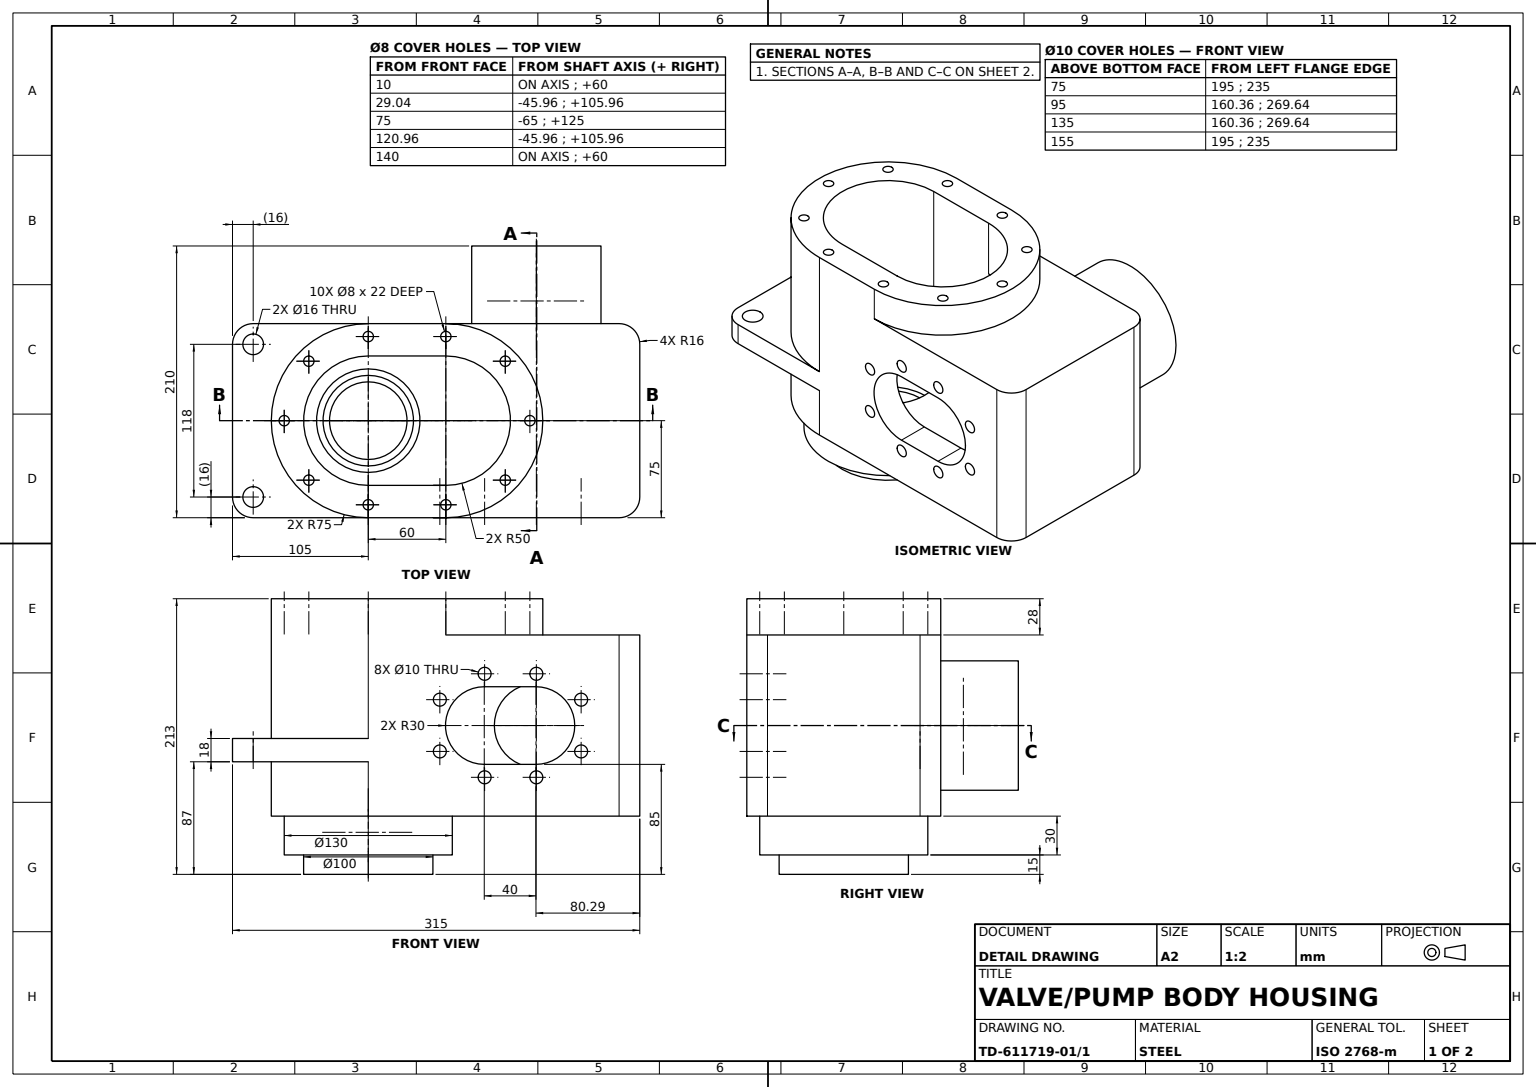
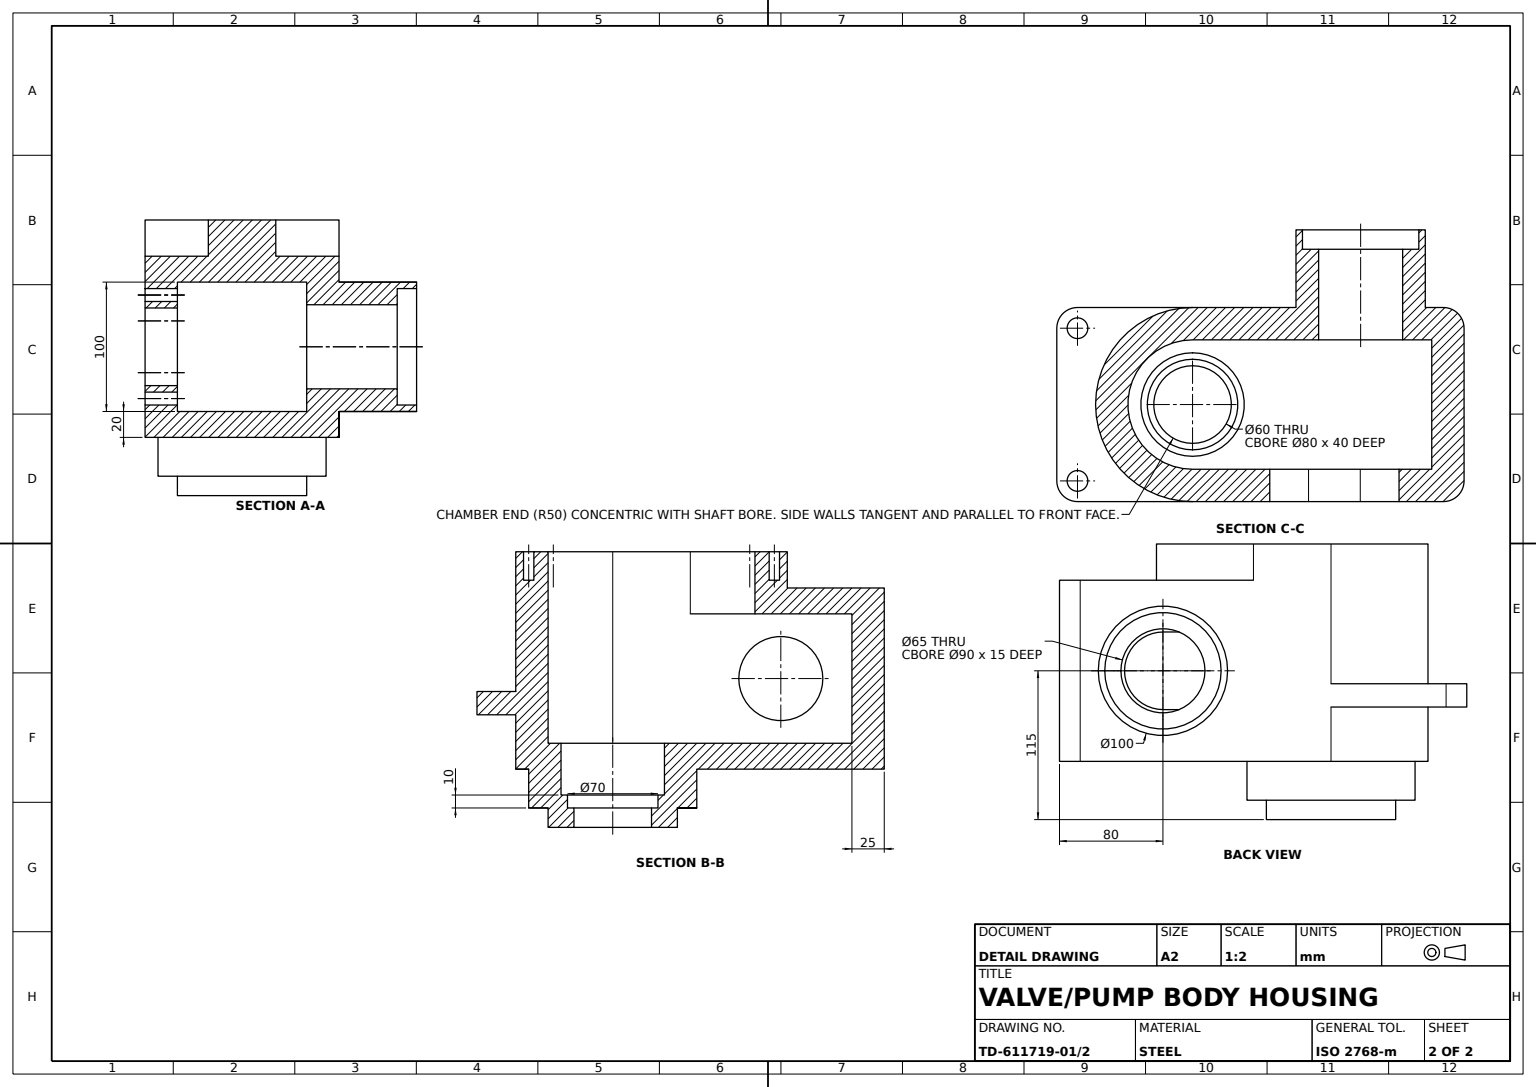
SolidWorks part; units mm, degrees
material "Plain Carbon Steel"
ref_plane "Front Plane" through (0, 0, 0) normal (0, 0, 1) x (1, 0, 0)
ref_plane "Top Plane" through (0, 0, 0) normal (0, 1, 0) x (1, 0, 0)
ref_plane "Right Plane" through (0, 0, 0) normal (1, 0, 0) x (0, 0, -1)
sketch "Base Boss Sketch" plane through (0, 0, 0) normal (0, 1, 0) x (1, 0, 0)
  circle A0 centre (0, 0) radius 50
  dimension "D1" = 100
extrude "Base Boss Ø100" add sketch "Base Boss Sketch" along normal blind 15
sketch "Bearing Boss Sketch" plane through (0, 15, 0) normal (0, 1, 0) x (1, 0, 0)
  circle A0 centre (0, 0) radius 65
  dimension "D1" = 130
extrude "Bearing Boss Ø130" add sketch "Bearing Boss Sketch" along normal blind 30
sketch "Housing Block Sketch" plane through (0, 45, 0) normal (0, 1, 0) x (1, 0, 0)
  line L0 (0, -75) -> (210, -75)
  line L1 (210, -75) -> (210, 75)
  line L2 (210, 75) -> (0, 75)
  arc A0 (0, 75) -> (0, -75) centre (0, 0) ccw
  dimension "D1" = 75
  dimension "D2" = 210
extrude "Housing Block 75x210" add sketch "Housing Block Sketch" along normal blind 168
sketch "Housing Recess Sketch" plane through (0, 213, 0) normal (0, 1, 0) x (1, 0, 0)
  line L1 (60, 75) -> (210, 75)
  line L2 (210, 75) -> (210, -75)
  line L3 (210, -75) -> (60, -75)
  arc A0 (60, -75) -> (60, 75) centre (60, 0) ccw
extrude "Housing Recess Cut" cut sketch "Housing Recess Sketch" against normal blind 28
ref_plane "Mounting Flange Plane" through (0, 87, 0) normal (0, -1, 0) x (-1, 0, 0)
sketch "Mounting Flange Sketch" plane through (0, 87, 0) normal (0, -1, 0) x (-1, 0, 0)
  line L0 (-210, -75) -> (-210, 75) construction
  line L2 (105, 0) -> (105, 75)
  line L3 (105, 75) -> (0, 75)
  line L4 (105, 0) -> (105, -75)
  line L5 (105, -75) -> (0, -75)
  arc A0 (0, -75) -> (0, 75) centre (0, 0) ccw
  dimension "D1" = 315
  dimension "D2" = 105
extrude "Mounting Flange" add sketch "Mounting Flange Sketch" against normal blind 18
sketch "Gear Cavity Sketch" plane through (0, 0, 75) normal (0, 0, 1) x (1, 0, 0)
  line L0 (90, 155) -> (130, 155) construction
  line L2 (90, 75) -> (130, 75) construction
  line L3 (-65, 15) -> (65, 15) construction
  arc A0 (130, 75) -> (130, 155) centre (130, 115) ccw construction
  arc A1 (90, 155) -> (90, 75) centre (90, 115) ccw construction
  circle A2 centre (130, 155) radius 5
  circle A3 centre (90, 155) radius 5
  circle A5 centre (164.641, 135) radius 5
  circle A6 centre (164.641, 95) radius 5
  circle A7 centre (130, 75) radius 5
  circle A8 centre (90, 75) radius 5
  circle A9 centre (55.359, 95) radius 5
  circle A10 centre (55.359, 135) radius 5
  dimension "D1" = 40
  dimension "D3" = 90
  dimension "D4" = 10
  dimension "D6" = 10
  dimension "D7" = 10
  dimension "D8" = 10
  dimension "D10" = 10
  dimension "D12" = 10
  dimension "D13" = 10
  dimension "D14" = 10
  dimension "D2" = 100
  dimension "D5" = 20
  dimension "D9" = 20
  dimension "D11" = 20
  dimension "D15" = 20
extrude "Gear Cavity Cut" cut sketch "Gear Cavity Sketch" against normal blind 94
sketch "Cavity Relief Sketch" plane through (0, 0, 75) normal (0, 0, 1) x (1, 0, 0)
  line L0 (89.7087, 145) -> (129.7087, 145)
  line L2 (89.7087, 85) -> (129.7087, 85)
  line L3 (-65, 45) -> (65, 45) construction
  line L4 (210, 185) -> (210, 45) construction
  arc A0 (129.7087, 85) -> (129.7087, 145) centre (129.7087, 115) ccw
  arc A1 (89.7087, 145) -> (89.7087, 85) centre (89.7087, 115) ccw
  dimension "D1" = 30
  dimension "D2" = 89.7087
  dimension "D4" = 80.2913
  dimension "D3" = 70
extrude "Cavity Relief Cut" cut sketch "Cavity Relief Sketch" against normal blind 94
sketch "Port Boss Sketch" plane through (0, 0, -75) normal (0, 0, -1) x (-1, 0, 0)
  circle A0 centre (-130, 115) radius 50
  dimension "D1" = 100
  dimension "D2" = 130
  dimension "D3" = 115
extrude "Port Boss Ø100" add sketch "Port Boss Sketch" along normal blind 60
sketch "Port Counterbore Sketch" plane through (0, 0, -135) normal (0, 0, -1) x (-1, 0, 0)
  circle A0 centre (-130, 115) radius 45
  dimension "D1" = 90
extrude "Port Counterbore Ø90" cut sketch "Port Counterbore Sketch" against normal blind 15
sketch "Port Bore Sketch" plane through (0, 0, -120) normal (0, 0, -1) x (-1, 0, 0)
  circle A0 centre (-130, 115) radius 32.5
  dimension "D1" = 65
extrude "Port Bore Ø65" cut sketch "Port Bore Sketch" against normal blind 150
ref_plane "Side Pocket Plane" through (0, 115, 0) normal (0, -1, 0) x (-1, 0, 0)
sketch "Side Pocket Sketch" plane through (0, 115, 0) normal (0, -1, 0) x (-1, 0, 0)
  line L0 (0, 50) -> (-185, 50)
  line L1 (-185, 50) -> (-185, -50)
  line L2 (-185, -50) -> (0, -50)
  arc A0 (0, -50) -> (0, 50) centre (0, 0) ccw
  dimension "D1" = 50
  dimension "D2" = 185
extrude "Side Pocket 50x185" cut sketch "Side Pocket Sketch" against normal mid plane 100
sketch "Base Bore Sketch" plane through (0, 0, 0) normal (0, -1, 0) x (1, 0, 0)
  circle A0 centre (0, 0) radius 30
  dimension "D1" = 60
extrude "Base Bore Ø60" cut sketch "Base Bore Sketch" against normal blind 15
sketch "Base Counterbore Sketch" plane through (0, 15, 0) normal (0, -1, 0) x (1, 0, 0)
  circle A0 centre (0, 0) radius 35
  dimension "D1" = 70
extrude "Base Counterbore Ø70" cut sketch "Base Counterbore Sketch" against normal blind 10
sketch "Shaft Bore Sketch" plane through (0, 25, 0) normal (0, -1, 0) x (1, 0, 0)
  circle A0 centre (0, 0) radius 40
  dimension "D1" = 80
extrude "Shaft Bore Ø80" cut sketch "Shaft Bore Sketch" against normal blind 119
sketch "Cover Bolt Holes Sketch" plane through (0, 213, 0) normal (0, 1, 0) x (1, 0, 0)
  line L1 (0, 65) -> (60, 65) construction
  line L2 (0, -65) -> (60, -65) construction
  arc A0 (0, 65) -> (0, -65) centre (0, 0) ccw construction
  arc A1 (60, -65) -> (60, 65) centre (60, 0) ccw construction
  circle A2 centre (125, 0) radius 4
  circle A3 centre (105.9619, 45.9619) radius 4
  circle A4 centre (105.9619, -45.9619) radius 4
  circle A5 centre (60, -65) radius 4
  circle A6 centre (0, -65) radius 4
  circle A7 centre (-45.9619, -45.9619) radius 4
  circle A8 centre (-45.9619, 45.9619) radius 4
  circle A9 centre (0, 65) radius 4
  circle A10 centre (60, 65) radius 4
  circle A11 centre (-65, 0) radius 4
  dimension "D1" = 8
  dimension "D2" = 8
  dimension "D3" = 8
  dimension "D4" = 8
  dimension "D5" = 8
  dimension "D6" = 8
  dimension "D7" = 8
  dimension "D8" = 8
  dimension "D9" = 8
  dimension "D10" = 8
  dimension "D11" = 45.9619
  dimension "D12" = 105.9619
  dimension "D13" = 125
  dimension "D14" = 105.9619
  dimension "D15" = 45.9619
  dimension "D16" = 45.9619
extrude "Cover Bolt Holes Ø8" cut sketch "Cover Bolt Holes Sketch" against normal blind 22
fillet "Flange Fillet R16 A" radius 16 1 edges at (-105, 96, 75)
fillet "Flange Fillet R16 B" radius 16 1 edges at (-105, 96, -75)
sketch "Flange Bolt Holes Sketch" plane through (0, 105, 0) normal (0, 1, 0) x (1, 0, 0)
  circle A0 centre (-89, 59) radius 8
  circle A1 centre (-89, -59) radius 8
  dimension "D1" = 16
  dimension "D2" = 16
extrude "Flange Bolt Holes Ø16" cut sketch "Flange Bolt Holes Sketch" against normal blind 91
sketch "Inner Slot Sketch" plane through (0, 213, 0) normal (0, 1, 0) x (1, 0, 0)
  line L0 (60, -50) -> (0, -50)
  line L1 (60, 50) -> (0, 50)
  arc A0 (0, 50) -> (0, -50) centre (0, 0) ccw
  arc A1 (60, -50) -> (60, 50) centre (60, 0) ccw
  dimension "D1" = 50
extrude "Inner Slot Cut" cut sketch "Inner Slot Sketch" against normal blind 91
fillet "Housing Fillet R16 A" radius 16 1 edges at (210, 115, -75)
fillet "Housing Fillet R16 B" radius 16 1 edges at (210, 115, 75)
